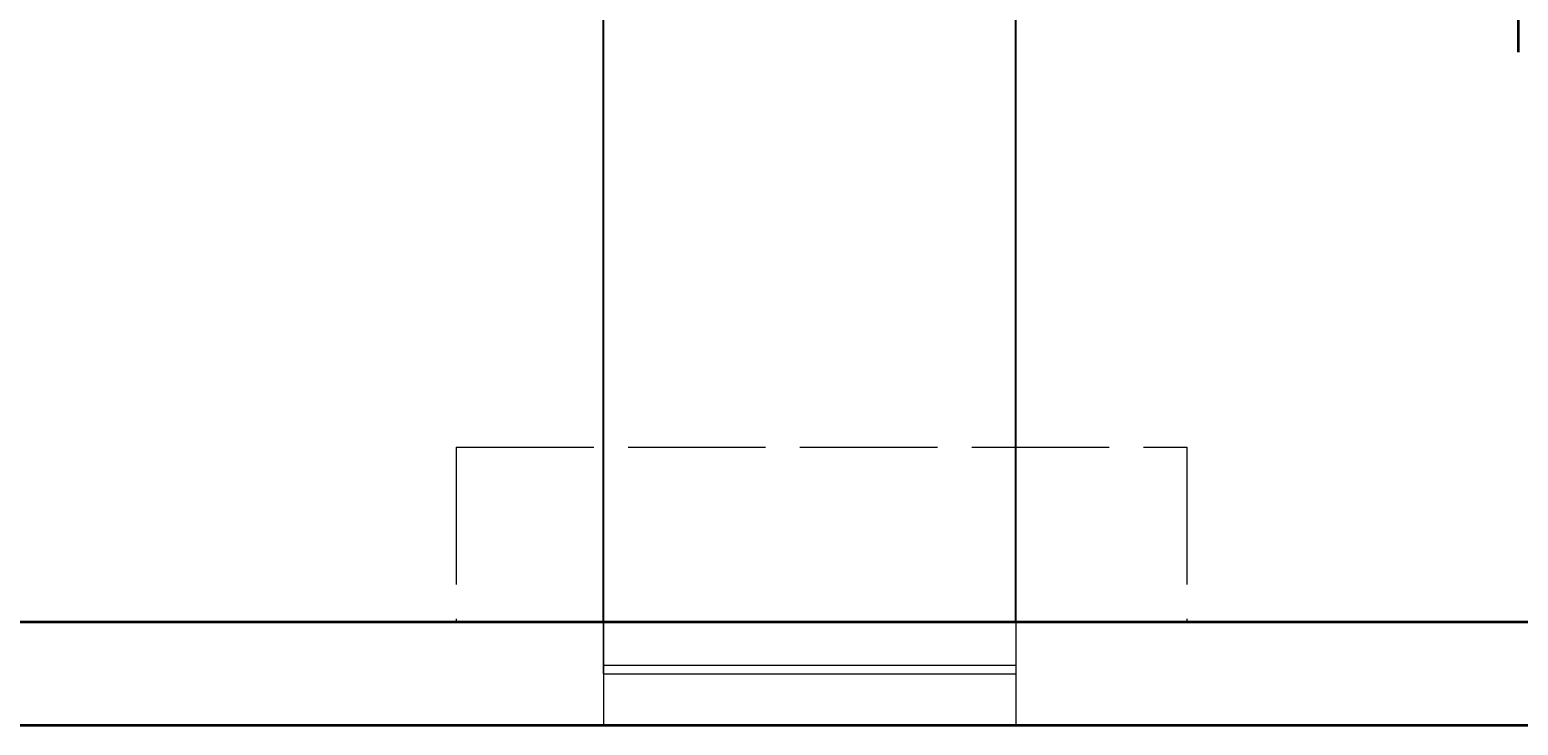
# Model space of a CAD drawing. Units: inches. Extents: x -61 to 1599, y -1316 to 257.
# Tile 75 of 204: x 406 to 536, y -626 to -565. Entities that reach past the tile are written whole.
import ezdxf

# ---------------------------------------------------------------- set-up
doc = ezdxf.new("R2010")
doc.units = ezdxf.units.IN
doc.header["$MEASUREMENT"] = 0
doc.linetypes.add('ACAD_ISO02W100', pattern=[15, 12, -3])
for name, color, linetype, lineweight in [('A-ANNO-DIMS', 2, 'Continuous', 18), ('A-FLOR-OVHD', 203, 'ACAD_ISO02W100', 13), ('WALLS', 4, 'Continuous', 35), ('WINDOWS', 220, 'Continuous', 18)]:
    doc.layers.add(name, color=color, linetype=linetype, lineweight=lineweight)
doc.styles.get("Standard").update_dxf_attribs({"font": 'arial.ttf'})
doc.dimstyles.get("Standard").update_dxf_attribs({"dimtxt": 0.18, "dimasz": 0.18, "dimexe": 0.18, "dimexo": 0.0625, "dimgap": 0.09, "dimtad": 0, "dimtih": 1, "dimtoh": 1, "dimdec": 0, "dimzin": 0, "dimdsep": 46, "dimlunit": 3, "dimtxsty": 'Standard', "dimcen": 0.09, "dimadec": 0, "dimazin": 0, "dimtfac": 1, "dimtdec": 0, "dimtofl": 0, "dimtmove": 0, "dimatfit": 3, "dimfxl": 1, "dimtolj": 1, "dimtzin": 0, "dimarcsym": 0})

# ---------------------------------------------------------------- blocks, each defined once
blk = doc.blocks.new('WIN-36IN')
for p, q in [((0, 4.5), (0, 9)), ((0, 9), (0, 0)), ((36, 9), (36, 0)), ((0, 5.26), (36, 5.26)), ((0, 4.5), (36, 4.5)), ((0, 4.5), (36, 4.5))]:
    blk.add_line(p, q)
blk = doc.blocks.new('*D703')
at = {"layer": 'A-ANNO-DIMS', "color": 0, "lineweight": -2, "transparency": 16777216}
for p, q in [((372.32, -616.88), (372.32, 257.46)), ((455.83, -616.88), (455.83, 257.46)), ((372.5, 257.28), (413.7, 257.28)), ((455.65, 257.28), (414.45, 257.28))]:
    blk.add_line(p, q, dxfattribs=at)
at = {"layer": 'A-ANNO-DIMS', "color": 0, "transparency": 16777216}
for points in [[(372.5, 257.31), (372.5, 257.25), (372.32, 257.28)], [(455.65, 257.31), (455.65, 257.25), (455.83, 257.28)]]:
    blk.add_solid(points, dxfattribs=at)
at = {"layer": 'DEFPOINTS', "color": 0, "transparency": 16777216}
for p in [(455.83, 257.28), (372.32, -616.94), (455.83, -616.94)]:
    blk.add_point(p, dxfattribs=at)
at = {"layer": 'A-ANNO-DIMS', "color": 0, "transparency": 16777216, "insert": (414.08, 257.28), "char_height": 0.18, "attachment_point": 5}
blk.add_mtext('\\A1;83.51', dxfattribs=at)
blk = doc.blocks.new('*D704')
at = {"layer": 'A-ANNO-DIMS', "color": 0, "lineweight": -2, "transparency": 16777216}
for p, q in [((491.83, -616.88), (491.83, 257.46)), ((544.7, -616.88), (544.7, 257.46)), ((492.01, 257.28), (517.87, 257.28)), ((544.52, 257.28), (518.66, 257.28))]:
    blk.add_line(p, q, dxfattribs=at)
at = {"layer": 'A-ANNO-DIMS', "color": 0, "transparency": 16777216}
for points in [[(492.01, 257.31), (492.01, 257.25), (491.83, 257.28)], [(544.52, 257.31), (544.52, 257.25), (544.7, 257.28)]]:
    blk.add_solid(points, dxfattribs=at)
at = {"layer": 'DEFPOINTS', "color": 0, "transparency": 16777216}
for p in [(544.7, 257.28), (491.83, -616.94), (544.7, -616.94)]:
    blk.add_point(p, dxfattribs=at)
at = {"layer": 'A-ANNO-DIMS', "color": 0, "transparency": 16777216, "insert": (518.27, 257.28), "char_height": 0.18, "attachment_point": 5}
blk.add_mtext('\\A1;52.87', dxfattribs=at)

msp = doc.modelspace()

# ---------------------------------------------------------------- linework, layer by layer
at = {"layer": 'A-FLOR-OVHD'}
for p, q in [((442.9886, -601.6522), (442.9886, -616.9446)), ((442.9886, -601.6522), (506.76, -601.6522)), ((506.76, -601.6522), (506.76, -616.9446))]:
    msp.add_line(p, q, dxfattribs=at)
at = {"layer": 'WALLS'}
for p, q in [((535.7028, -441.3229), (535.7028, -567.169)), ((544.7028, -616.9446), (14.7028, -616.9446)), ((403.7028, -625.9446), (535.7028, -625.9446)), ((535.7028, -625.9446), (544.7028, -625.9446))]:
    msp.add_line(p, q, dxfattribs=at)

# ---------------------------------------------------------------- block references
at = {"layer": 'WINDOWS'}
msp.add_blockref('WIN-36IN', (455.8326, -625.9447), dxfattribs=at)

# ---------------------------------------------------------------- dimensions: what is measured, and where the dimension line sits
at = {"layer": 'A-ANNO-DIMS'}
for base, p1, p2, picture, middle in [((455.8327, 257.2771), (372.3201, -616.9446), (455.8327, -616.9446), '*D703', (414.0764, 257.2771)), ((544.7028, 257.2771), (491.8327, -616.9446), (544.7028, -616.9446), '*D704', (518.2677, 257.2771))]:
    dim = msp.add_linear_dim(base=base, p1=p1, p2=p2, dimstyle='Standard', override={"dimdec": 2, "dimlfac": 1, "dimrnd": 0, "dimzin": 0, "dimdsep": 46, "dimlunit": 2}, dxfattribs=at)
    dim.commit()
    dim.dimension.update_dxf_attribs({"geometry": picture, "text_midpoint": middle})

doc.saveas('drawing.dxf')
